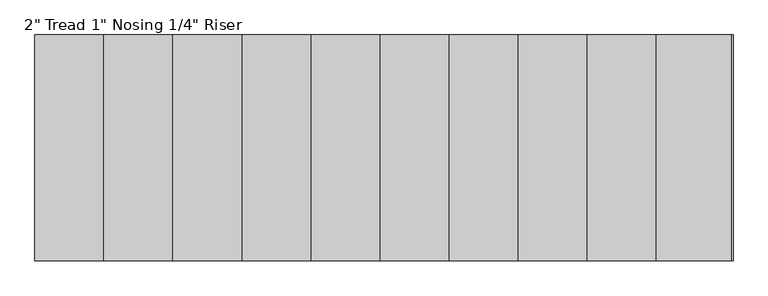
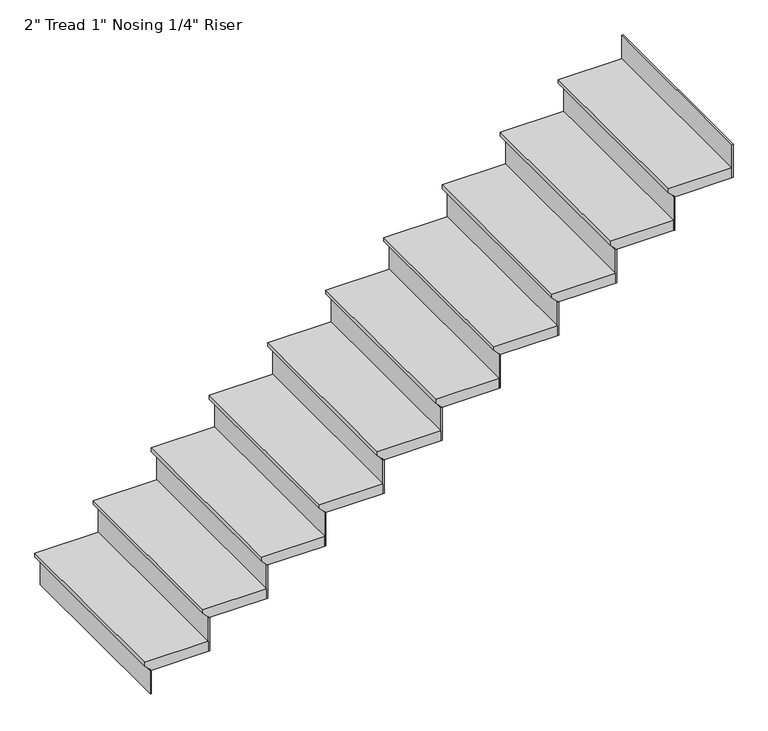
"""IFC4 building model written with IfcOpenShell, lengths in millimetres: stair flight geometry."""

from ifc_helpers import new_model, si_unit, frame, origin, origin_with_axes, place, context, project, spatial, polyline, outline, extrude, source, transform, mapped, element, save


def stair_flight_ef839ef7(model_context):
    return source(origin(), model_context, "Body", "SweptSolid", [
        extrude(outline(polyline([(169.3333333, -12731.56961), (169.3333333, -13036.36961), (150.2833333, -13036.36961), (124.8833333, -13010.96961), (118.5333333, -13010.96961), (118.5333333, -12731.56961), (169.3333333, -12731.56961)])), frame((0.0, 6598.3146616, 0.0), z_axis=(0.0, 1.0, 0.0), x_axis=(0.0, 0.0, 1.0)), (0.0, 0.0, 1.0), 914.4),
        extrude(outline(polyline([(-13004.61961, 6598.3146616), (-13010.96961, 6598.3146616), (-13010.96961, 7512.7146616), (-13004.61961, 7512.7146616), (-13004.61961, 6598.3146616)])), origin_with_axes(), (0.0, 0.0, 1.0), 118.5333333),
        extrude(outline(polyline([(-12725.21961, 6598.3146616), (-12731.56961, 6598.3146616), (-12731.56961, 7512.7146616), (-12725.21961, 7512.7146616), (-12725.21961, 6598.3146616)])), frame((0.0, 0.0, 118.5333333), z_axis=(0.0, 0.0, 1.0), x_axis=(1.0, 0.0, 0.0)), (0.0, 0.0, 1.0), 169.3333333),
        extrude(outline(polyline([(338.6666667, -12452.16961), (338.6666667, -12756.96961), (319.6166667, -12756.96961), (294.2166667, -12731.56961), (287.8666667, -12731.56961), (287.8666667, -12452.16961), (338.6666667, -12452.16961)])), frame((0.0, 6598.3146616, 0.0), z_axis=(0.0, 1.0, 0.0), x_axis=(0.0, 0.0, 1.0)), (0.0, 0.0, 1.0), 914.4),
        extrude(outline(polyline([(-12445.81961, 6598.3146616), (-12452.16961, 6598.3146616), (-12452.16961, 7512.7146616), (-12445.81961, 7512.7146616), (-12445.81961, 6598.3146616)])), frame((0.0, 0.0, 287.8666667), z_axis=(0.0, 0.0, 1.0), x_axis=(1.0, 0.0, 0.0)), (0.0, 0.0, 1.0), 169.3333333),
        extrude(outline(polyline([(508.0, -12172.76961), (508.0, -12477.56961), (488.95, -12477.56961), (463.55, -12452.16961), (457.2, -12452.16961), (457.2, -12172.76961), (508.0, -12172.76961)])), frame((0.0, 6598.3146616, 0.0), z_axis=(0.0, 1.0, 0.0), x_axis=(0.0, 0.0, 1.0)), (0.0, 0.0, 1.0), 914.4),
        extrude(outline(polyline([(-12166.41961, 6598.3146616), (-12172.76961, 6598.3146616), (-12172.76961, 7512.7146616), (-12166.41961, 7512.7146616), (-12166.41961, 6598.3146616)])), frame((0.0, 0.0, 457.2), z_axis=(0.0, 0.0, 1.0), x_axis=(1.0, 0.0, 0.0)), (0.0, 0.0, 1.0), 169.3333333),
        extrude(outline(polyline([(677.3333333, -11893.36961), (677.3333333, -12198.16961), (658.2833333, -12198.16961), (632.8833333, -12172.76961), (626.5333333, -12172.76961), (626.5333333, -11893.36961), (677.3333333, -11893.36961)])), frame((0.0, 6598.3146616, 0.0), z_axis=(0.0, 1.0, 0.0), x_axis=(0.0, 0.0, 1.0)), (0.0, 0.0, 1.0), 914.4),
        extrude(outline(polyline([(-11887.01961, 6598.3146616), (-11893.36961, 6598.3146616), (-11893.36961, 7512.7146616), (-11887.01961, 7512.7146616), (-11887.01961, 6598.3146616)])), frame((0.0, 0.0, 626.5333333), z_axis=(0.0, 0.0, 1.0), x_axis=(1.0, 0.0, 0.0)), (0.0, 0.0, 1.0), 169.3333333),
        extrude(outline(polyline([(846.6666667, -11613.96961), (846.6666667, -11918.76961), (827.6166667, -11918.76961), (802.2166667, -11893.36961), (795.8666667, -11893.36961), (795.8666667, -11613.96961), (846.6666667, -11613.96961)])), frame((0.0, 6598.3146616, 0.0), z_axis=(0.0, 1.0, 0.0), x_axis=(0.0, 0.0, 1.0)), (0.0, 0.0, 1.0), 914.4),
        extrude(outline(polyline([(-11607.61961, 6598.3146616), (-11613.96961, 6598.3146616), (-11613.96961, 7512.7146616), (-11607.61961, 7512.7146616), (-11607.61961, 6598.3146616)])), frame((0.0, 0.0, 795.8666667), z_axis=(0.0, 0.0, 1.0), x_axis=(1.0, 0.0, 0.0)), (0.0, 0.0, 1.0), 169.3333333),
        extrude(outline(polyline([(1016.0, -11334.56961), (1016.0, -11639.36961), (996.95, -11639.36961), (971.55, -11613.96961), (965.2, -11613.96961), (965.2, -11334.56961), (1016.0, -11334.56961)])), frame((0.0, 6598.3146616, 0.0), z_axis=(0.0, 1.0, 0.0), x_axis=(0.0, 0.0, 1.0)), (0.0, 0.0, 1.0), 914.4),
        extrude(outline(polyline([(-11328.21961, 6598.3146616), (-11334.56961, 6598.3146616), (-11334.56961, 7512.7146616), (-11328.21961, 7512.7146616), (-11328.21961, 6598.3146616)])), frame((0.0, 0.0, 965.2), z_axis=(0.0, 0.0, 1.0), x_axis=(1.0, 0.0, 0.0)), (0.0, 0.0, 1.0), 169.3333333),
        extrude(outline(polyline([(1185.3333333, -11055.16961), (1185.3333333, -11359.96961), (1166.2833333, -11359.96961), (1140.8833333, -11334.56961), (1134.5333333, -11334.56961), (1134.5333333, -11055.16961), (1185.3333333, -11055.16961)])), frame((0.0, 6598.3146616, 0.0), z_axis=(0.0, 1.0, 0.0), x_axis=(0.0, 0.0, 1.0)), (0.0, 0.0, 1.0), 914.4),
        extrude(outline(polyline([(-11048.81961, 6598.3146616), (-11055.16961, 6598.3146616), (-11055.16961, 7512.7146616), (-11048.81961, 7512.7146616), (-11048.81961, 6598.3146616)])), frame((0.0, 0.0, 1134.5333333), z_axis=(0.0, 0.0, 1.0), x_axis=(1.0, 0.0, 0.0)), (0.0, 0.0, 1.0), 169.3333333),
        extrude(outline(polyline([(1354.6666667, -10775.76961), (1354.6666667, -11080.56961), (1335.6166667, -11080.56961), (1310.2166667, -11055.16961), (1303.8666667, -11055.16961), (1303.8666667, -10775.76961), (1354.6666667, -10775.76961)])), frame((0.0, 6598.3146616, 0.0), z_axis=(0.0, 1.0, 0.0), x_axis=(0.0, 0.0, 1.0)), (0.0, 0.0, 1.0), 914.4),
        extrude(outline(polyline([(-10769.41961, 6598.3146616), (-10775.76961, 6598.3146616), (-10775.76961, 7512.7146616), (-10769.41961, 7512.7146616), (-10769.41961, 6598.3146616)])), frame((0.0, 0.0, 1303.8666667), z_axis=(0.0, 0.0, 1.0), x_axis=(1.0, 0.0, 0.0)), (0.0, 0.0, 1.0), 169.3333333),
        extrude(outline(polyline([(1524.0, -10496.36961), (1524.0, -10801.16961), (1504.95, -10801.16961), (1479.55, -10775.76961), (1473.2, -10775.76961), (1473.2, -10496.36961), (1524.0, -10496.36961)])), frame((0.0, 6598.3146616, 0.0), z_axis=(0.0, 1.0, 0.0), x_axis=(0.0, 0.0, 1.0)), (0.0, 0.0, 1.0), 914.4),
        extrude(outline(polyline([(-10490.01961, 6598.3146616), (-10496.36961, 6598.3146616), (-10496.36961, 7512.7146616), (-10490.01961, 7512.7146616), (-10490.01961, 6598.3146616)])), frame((0.0, 0.0, 1473.2), z_axis=(0.0, 0.0, 1.0), x_axis=(1.0, 0.0, 0.0)), (0.0, 0.0, 1.0), 169.3333333),
        extrude(outline(polyline([(-10210.61961, 6598.3146616), (-10216.96961, 6598.3146616), (-10216.96961, 7512.7146616), (-10210.61961, 7512.7146616), (-10210.61961, 6598.3146616)])), frame((0.0, 0.0, 1642.5333333), z_axis=(0.0, 0.0, 1.0), x_axis=(1.0, 0.0, 0.0)), (0.0, 0.0, 1.0), 169.3333333),
        extrude(outline(polyline([(1693.3333333, -10216.96961), (1693.3333333, -10521.76961), (1674.2833333, -10521.76961), (1648.8833333, -10496.36961), (1642.5333333, -10496.36961), (1642.5333333, -10216.96961), (1693.3333333, -10216.96961)])), frame((0.0, 6598.3146616, 0.0), z_axis=(0.0, 1.0, 0.0), x_axis=(0.0, 0.0, 1.0)), (0.0, 0.0, 1.0), 914.4),
    ])


if __name__ == "__main__":
    model = new_model("IFC4")
    model_context = context("Model", 3, world=origin())
    ifc_project = project(units=[si_unit("LENGTHUNIT", "METRE", prefix="MILLI")], contexts=[model_context])
    site = spatial("IfcSite", under=ifc_project)
    building = spatial("IfcBuilding", under=site)
    placement = place(None, origin())
    stair_flight_shape = stair_flight_ef839ef7(model_context)
    element("IfcStairFlight", 1, ObjectType="2\" Tread 1\" Nosing 1/4\" Riser", at=placement, inside=building, context=model_context, shape_type="MappedRepresentation", body=[
        mapped(stair_flight_shape, transform((0.0, 0.0, 0.0), x_axis=(1.0, 0.0, 0.0), y_axis=(0.0, 1.0, 0.0), z_axis=(0.0, 0.0, 1.0))),
    ])
    save(model, "model.ifc")
